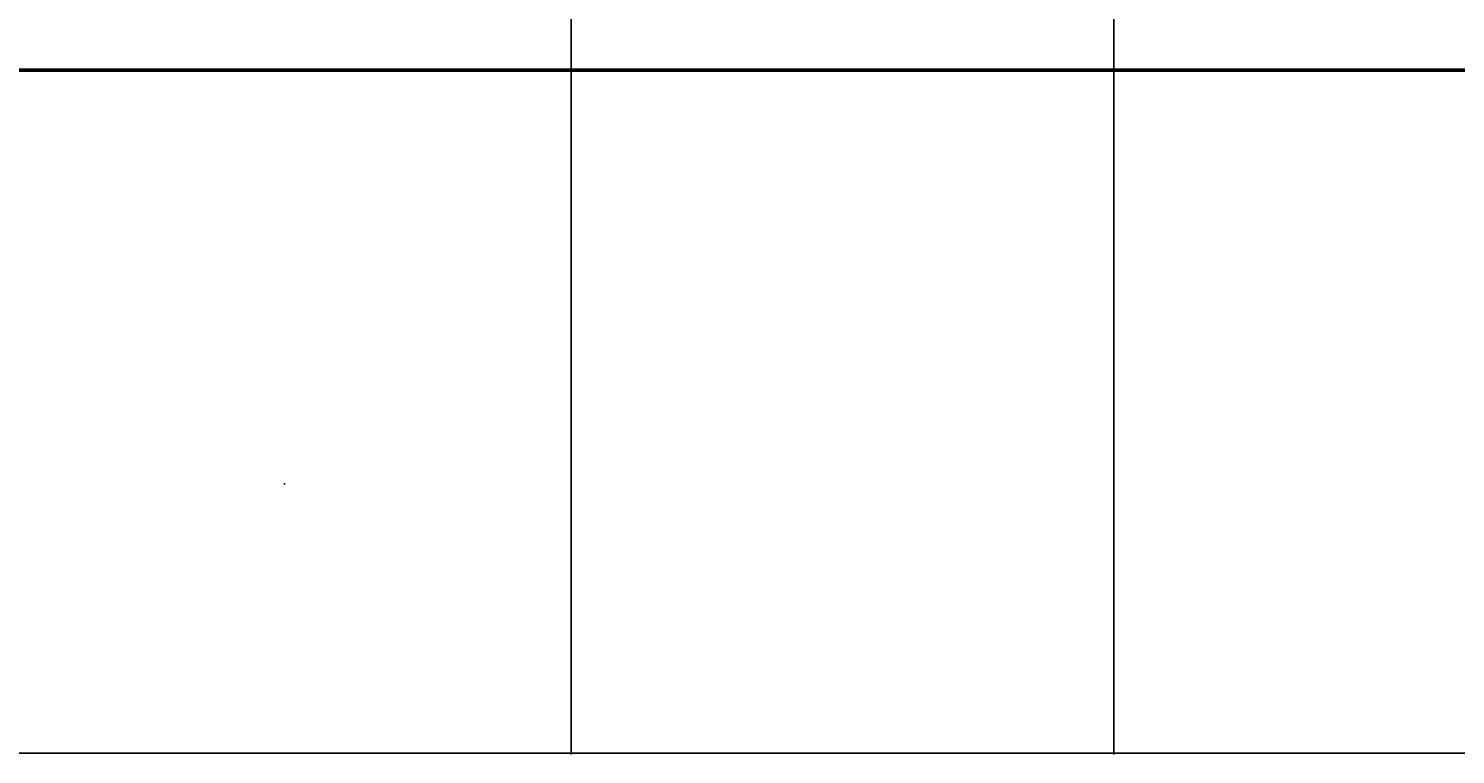
# Model space of a CAD drawing. Units: inches. Extents: x 5375 to 6084, y 16106 to 17259.
# Tile 4 of 32: x 5624 to 5844, y 16106 to 16219. Entities that reach past the tile are written whole.
import ezdxf

# ---------------------------------------------------------------- set-up
doc = ezdxf.new("R2010")
doc.units = ezdxf.units.IN
doc.layers.add('A-ANNO-DIMS', color=2, linetype='Continuous', lineweight=18)
doc.layers.add('WALL', color=6, linetype='Continuous', lineweight=50)
doc.styles.get("Standard").update_dxf_attribs({"font": 'arial.ttf'})
doc.dimstyles.get("Standard").update_dxf_attribs({"dimtxt": 0.18, "dimasz": 0.18, "dimexe": 0.18, "dimexo": 0.0625, "dimgap": 0.09, "dimtad": 0, "dimtih": 1, "dimtoh": 1, "dimdec": 4, "dimzin": 0, "dimdsep": 46, "dimtxsty": 'Standard', "dimcen": 0.09, "dimadec": 0, "dimazin": 0, "dimtfac": 1, "dimtdec": 4, "dimtofl": 0, "dimtmove": 0, "dimatfit": 3, "dimfxl": 1, "dimtolj": 1, "dimtzin": 0, "dimarcsym": 0})

# ---------------------------------------------------------------- blocks, each defined once
blk = doc.blocks.new('*D30')
at = {"layer": 'A-ANNO-DIMS', "color": 0, "lineweight": -2, "transparency": 16777216}
for p, q in [((5470.62, 16212.32), (5470.62, 16106.48)), ((6031.62, 16212.32), (6031.62, 16106.48)), ((5470.8, 16106.66), (5750.85, 16106.66)), ((6031.44, 16106.66), (5751.39, 16106.66))]:
    blk.add_line(p, q, dxfattribs=at)
at = {"layer": 'A-ANNO-DIMS', "color": 0, "transparency": 16777216}
for points in [[(5470.8, 16106.69), (5470.8, 16106.63), (5470.62, 16106.66)], [(6031.44, 16106.69), (6031.44, 16106.63), (6031.62, 16106.66)]]:
    blk.add_solid(points, dxfattribs=at)
at = {"layer": 'Defpoints', "color": 0, "transparency": 16777216}
for p in [(5470.62, 16212.38), (6031.62, 16212.38), (6031.62, 16106.66)]:
    blk.add_point(p, dxfattribs=at)
at = {"layer": 'A-ANNO-DIMS', "color": 0, "transparency": 16777216, "insert": (5751.12, 16106.66), "char_height": 0.18, "attachment_point": 5}
blk.add_mtext('\\A1;561', dxfattribs=at)
blk = doc.blocks.new('*D38')
at = {"layer": 'A-ANNO-DIMS', "color": 0, "lineweight": -2, "transparency": 16777216}
for p, q in [((5791.62, 16513.52), (5791.62, 16106.48)), ((5707.62, 16507.52), (5707.62, 16106.48)), ((5707.8, 16106.66), (5749.4, 16106.66)), ((5791.44, 16106.66), (5749.84, 16106.66))]:
    blk.add_line(p, q, dxfattribs=at)
at = {"layer": 'A-ANNO-DIMS', "color": 0, "transparency": 16777216}
for points in [[(5707.8, 16106.69), (5707.8, 16106.63), (5707.62, 16106.66)], [(5791.44, 16106.69), (5791.44, 16106.63), (5791.62, 16106.66)]]:
    blk.add_solid(points, dxfattribs=at)
at = {"layer": 'Defpoints', "color": 0, "transparency": 16777216}
for p in [(5791.62, 16513.58), (5707.62, 16507.58), (5791.62, 16106.66)]:
    blk.add_point(p, dxfattribs=at)
at = {"layer": 'A-ANNO-DIMS', "color": 0, "transparency": 16777216, "insert": (5749.62, 16106.66), "char_height": 0.18, "attachment_point": 5}
blk.add_mtext('\\A1;84', dxfattribs=at)
blk = doc.blocks.new('*D51')
at = {"layer": 'A-ANNO-DIMS', "color": 0, "lineweight": -2, "transparency": 16777216}
for p, q in [((5820.47, 16344.39), (5761.62, 16271.02)), ((5820.65, 16344.39), (5820.47, 16344.39)), ((5663.14, 16148.34), (5663.32, 16148.34)), ((5663.23, 16148.25), (5663.23, 16148.43))]:
    blk.add_line(p, q, dxfattribs=at)
at = {"layer": 'A-ANNO-DIMS', "color": 0, "transparency": 16777216}
blk.add_solid([(5761.59, 16271.03), (5761.64, 16271), (5761.5, 16270.88)], dxfattribs=at)
at = {"layer": 'Defpoints', "color": 0, "transparency": 16777216}
for p in [(5761.5, 16270.88), (5663.23, 16148.34)]:
    blk.add_point(p, dxfattribs=at)
at = {"layer": 'A-ANNO-DIMS', "color": 0, "transparency": 16777216, "insert": (5821.2, 16344.39), "char_height": 0.18, "attachment_point": 5}
blk.add_mtext('\\A1;R157.07', dxfattribs=at)

msp = doc.modelspace()

# ---------------------------------------------------------------- linework, layer by layer
at = {"layer": 'WALL'}
msp.add_line((5470.6199, 16212.3785), (6031.6199, 16212.3785), dxfattribs=at)

# ---------------------------------------------------------------- dimensions: what is measured, and where the dimension line sits
at = {"layer": 'A-ANNO-DIMS'}
for base, p1, p2, picture, middle in [((5791.6199, 16106.6631), (5707.6199, 16507.5793), (5791.6199, 16513.5793), '*D38', (5749.6199, 16106.6631)), ((6031.6199, 16106.6631), (5470.6199, 16212.3785), (6031.6199, 16212.3785), '*D30', (5751.1199, 16106.6631))]:
    dim = msp.add_linear_dim(base=base, p1=p1, p2=p2, dimstyle='Standard', override={"dimdec": 0, "dimlfac": 1, "dimrnd": 0, "dimzin": 0, "dimdsep": 46, "dimlunit": 2}, dxfattribs=at)
    dim.commit()
    dim.dimension.update_dxf_attribs({"geometry": picture, "text_midpoint": middle})
dim = msp.add_radius_dim(center=(5663.2298, 16148.3446), mpoint=(5761.504, 16270.8753), dimstyle='Standard', override={"dimdec": 2, "dimlfac": 1, "dimrnd": 0, "dimzin": 0, "dimdsep": 46, "dimlunit": 2}, dxfattribs=at)
dim.commit()
dim.dimension.update_dxf_attribs({"geometry": '*D51', "text_midpoint": (5821.1984, 16344.3937), "dimtype": 164})

doc.saveas('drawing.dxf')
